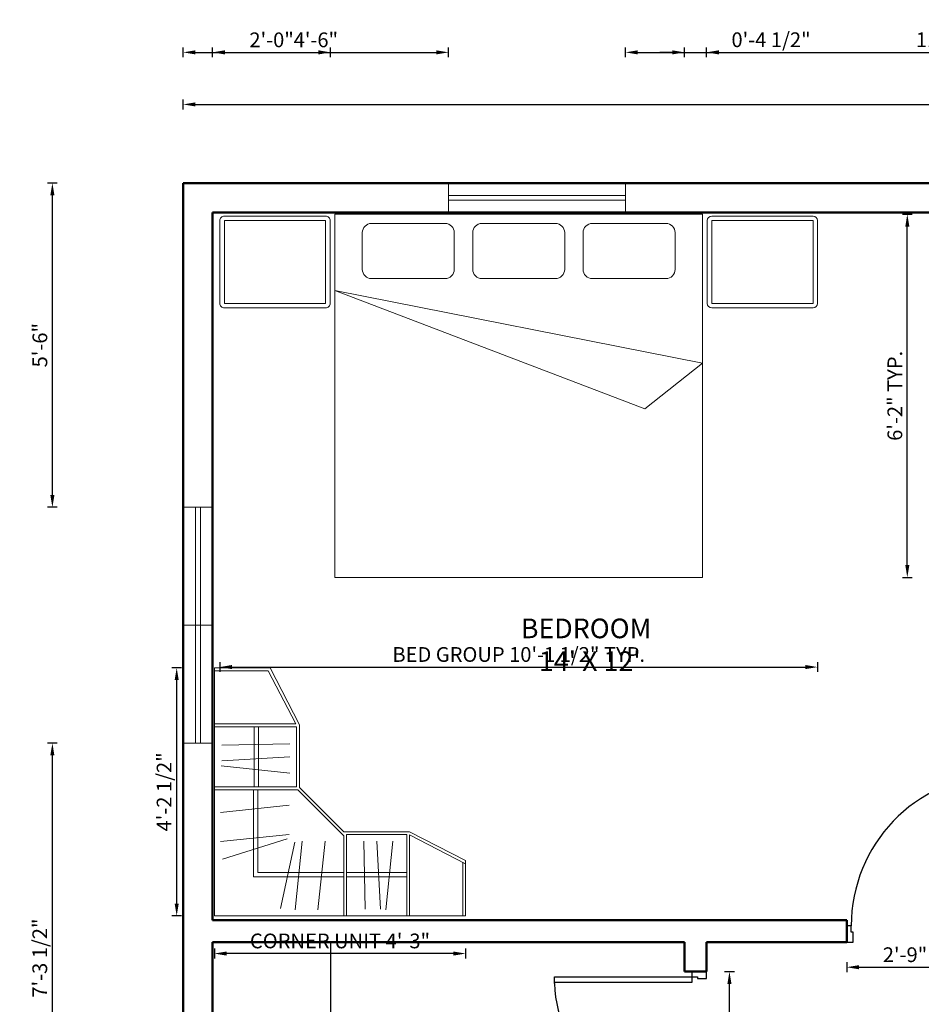
# Model space of a CAD drawing. Units: inches. Extents: x 1961 to 3038, y 800 to 1438.
# Tile 11 of 13: x 2592 to 2775, y 1148 to 1348. Entities that reach past the tile are written whole.
import ezdxf

# ---------------------------------------------------------------- set-up
doc = ezdxf.new("R2010")
doc.units = ezdxf.units.IN
for name, color, linetype, lineweight in [('A-ANNO-DIMS', 2, 'Continuous', 18), ('A-AREA-IDEN', 7, 'Continuous', 25), ('A-DOOR', 3, 'Continuous', 25), ('A-FLOR-CASE', 8, 'Continuous', 25), ('A-FURN', 8, 'Continuous', 18), ('A-GLAZ', 4, 'Continuous', 18), ('A-WALL', 7, 'Continuous', 50)]:
    doc.layers.add(name, color=color, linetype=linetype, lineweight=lineweight)
doc.styles.get("Standard").update_dxf_attribs({"font": 'arial.ttf'})
doc.dimstyles.new('ISO-25', dxfattribs={"dimtxt": 3, "dimasz": 2.5, "dimexe": 1, "dimexo": 1, "dimtad": 1, "dimdec": 4, "dimlunit": 4, "dimtxsty": 'Standard', "dimcen": 2.5, "dimadec": 0, "dimazin": 0, "dimtfac": 1, "dimtdec": 4, "dimtmove": 0, "dimatfit": 3, "dimfxl": 1, "dimfxlon": 1, "dimarcsym": 0})

# ---------------------------------------------------------------- blocks, each defined once
blk = doc.blocks.new('door 26')
for p, q in [((2685.19, 1125.64), (2685.19, 1127.01)), ((2685.19, 1127.01), (2713.13, 1127.01)), ((2713.13, 1128.04), (2713.13, 1125.8)), ((2713.13, 1127.01), (2714.34, 1127.01)), ((2714.34, 1127.01), (2714.34, 1126.64)), ((2714.34, 1126.64), (2716.17, 1126.64)), ((2716.17, 1126.64), (2716.17, 1128.04)), ((2713.13, 1125.8), (2685.19, 1125.8))]:
    blk.add_line(p, q)
blk.add_lwpolyline([(2716.17, 1098.04), (2716.17, 1099.26), (2714.34, 1099.26), (2714.34, 1098.89), (2713.13, 1098.89), (2713.13, 1098.04)])
blk.add_arc((2713.13, 1126.85), 27.97, 182.4896, 270)
blk = doc.blocks.new('A$C793B20D3')
for p, q in [((0.575, 1.9405), (0.025, 1.9405)), ((0.025, 1.9405), (0.025, 1.4905)), ((0.575, 1.4905), (0.575, 1.9405)), ((0.625, 0), (0.625, 1.975)), ((2.625, 1.975), (0.625, 1.975)), ((2.625, 0), (2.625, 1.975)), ((2.65, 1.4905), (2.65, 1.9405)), ((2.675, 1.9655), (3.225, 1.9655)), ((3.25, 1.9405), (3.25, 1.4905)), ((0.775, 1.675), (0.775, 1.875)), ((0.825, 1.925), (1.225, 1.925)), ((1.275, 1.675), (1.275, 1.875)), ((1.375, 1.675), (1.375, 1.875)), ((1.425, 1.925), (1.825, 1.925)), ((1.875, 1.675), (1.875, 1.875)), ((1.975, 1.675), (1.975, 1.875)), ((2.025, 1.925), (2.425, 1.925)), ((2.475, 1.675), (2.475, 1.875)), ((0.825, 1.625), (1.225, 1.625)), ((1.425, 1.625), (1.825, 1.625)), ((2.025, 1.625), (2.425, 1.625)), ((0.6256, 1.5604), (2.3107, 0.9169)), ((0.6256, 1.5604), (2.625, 1.1646)), ((0.025, 1.4905), (0.575, 1.4905)), ((3.225, 1.4655), (2.675, 1.4655)), ((2.3107, 0.9169), (2.625, 1.1646)), ((2.625, 0), (0.625, 0))]:
    blk.add_line(p, q)
at = {"flags": 128}
blk.add_lwpolyline([(0, 1.9405), (0, 1.4905, 0.414214), (0.025, 1.4655), (0.575, 1.4655, 0.414214), (0.6, 1.4905), (0.6, 1.9405, 0.414214), (0.575, 1.9655), (0.025, 1.9655, 0.414214)], format="xyb", close=True, dxfattribs=at)
blk.add_lwpolyline([(3.225, 1.9405), (3.225, 1.4905), (2.675, 1.4905), (2.675, 1.9405)], close=True)
for centre, radius, start, end in [((2.675, 1.9405), 0.025, 90, 180), ((3.225, 1.9405), 0.025, 0, 90), ((0.825, 1.875), 0.05, 90, 180), ((1.225, 1.875), 0.05, 0, 90), ((1.425, 1.875), 0.05, 90, 180), ((1.825, 1.875), 0.05, 0, 90), ((2.025, 1.875), 0.05, 90, 180), ((2.425, 1.875), 0.05, 0, 90), ((0.825, 1.675), 0.05, 180, 270), ((1.225, 1.675), 0.05, 270, 0), ((1.425, 1.675), 0.05, 180, 270), ((1.825, 1.675), 0.05, 270, 0), ((2.025, 1.675), 0.05, 180, 270), ((2.425, 1.675), 0.05, 270, 0), ((2.675, 1.4905), 0.025, 180, 270), ((3.225, 1.4905), 0.025, 270, 0)]:
    blk.add_arc(centre, radius, start, end)
blk = doc.blocks.new('A$C379C348A')
for p, q in [((1186.4, 1363.9), (1396.2, 1771)), ((1396.2, 1771), (1793.4, 1771)), ((1793.4, 1771), (1793.4, 0)), ((1212.5, 1371), (1408.4, 1751)), ((1408.4, 1751), (1793.4, 1751)), ((1186.4, 917.4), (1186.4, 1363.9)), ((1206.4, 1351), (1793.4, 1351)), ((1206.4, 921), (1206.4, 1351)), ((1212.5, 1371), (1793.4, 1371)), ((1479, 921.6), (1479, 1351.6)), ((1509.8, 921.6), (1509.8, 1351.6)), ((1255.5, 1228.5), (1740.8, 1219.3)), ((1740.8, 1108.3), (1255.5, 1136)), ((1255.5, 1020.4), (1745.4, 1071.2)), ((870, 601), (1186.4, 917.4)), ((1206.4, 921), (1793.4, 921)), ((870, 572.7), (1198.3, 901)), ((1198.3, 901), (1793.4, 901)), ((1483.9, 901), (1484.1, 309.1)), ((1514.7, 901), (1514.9, 278.3)), ((1260.4, 789.5), (1750.4, 738.8)), ((0, 394.8), (400, 601)), ((0, 372.3), (400, 578.5)), ((850, 601), (400, 601)), ((400, 578.5), (400, 0)), ((420, 581), (420, 0)), ((850, 581), (420, 581)), ((850, 601), (870, 601)), ((850, 581), (850, 0)), ((870, 572.7), (870, 0)), ((1260.5, 581.2), (1750.5, 530.6)), ((518.8, 532.6), (569.6, 42.7)), ((606.7, 47.3), (634.4, 532.6)), ((726.9, 532.6), (717.7, 47.3)), ((1003.7, 532.6), (1054.5, 42.7)), ((1166.2, 532.6), (1217.1, 42.7)), ((1321.2, 51.6), (1217.9, 526.5)), ((1736.6, 405.8), (1272.7, 550.9)), ((0, 394.8), (0, 0)), ((20, 382.7), (20, 0)), ((420, 309.1), (850, 309.1)), ((870, 309.1), (1484.1, 309.1)), ((420, 278.3), (850, 278.3)), ((870, 278.3), (1514.9, 278.3)), ((0, 0), (1793.4, 0))]:
    blk.add_line(p, q)
blk = doc.blocks.new('*D25')
at = {"layer": 'A-ANNO-DIMS', "color": 0, "lineweight": -2, "transparency": 16777216}
for p, q in [((2624.77, 1329.92), (2624.77, 1331.92)), ((2627.27, 1330.92), (3006.27, 1330.92)), ((3008.77, 1329.92), (3008.77, 1331.92))]:
    blk.add_line(p, q, dxfattribs=at)
at = {"layer": 'A-ANNO-DIMS', "color": 0, "transparency": 16777216}
for points in [[(2627.27, 1331.34), (2627.27, 1330.51), (2624.77, 1330.92)], [(3006.27, 1331.34), (3006.27, 1330.51), (3008.77, 1330.92)]]:
    blk.add_solid(points, dxfattribs=at)
at = {"layer": 'Defpoints', "color": 0, "transparency": 16777216}
for p in [(3008.77, 1330.92), (2624.77, 1314.92), (3008.77, 1314.92)]:
    blk.add_point(p, dxfattribs=at)
at = {"layer": 'A-ANNO-DIMS', "color": 0, "transparency": 16777216, "insert": (2816.77, 1333.08), "char_height": 3, "attachment_point": 5}
blk.add_mtext("32'", dxfattribs=at)
blk = doc.blocks.new('WIN-36IN')
for p, q in [((0, 36), (6, 36)), ((2.5, 36), (2.5, 0)), ((3.5, 36), (3.5, 0)), ((0, 0), (6, 0))]:
    blk.add_line(p, q)
blk = doc.blocks.new('WIN-48IN-MULLION')
for p, q in [((6, 48), (0, 48)), ((2.5, 48), (2.5, 0)), ((3.5, 48), (3.5, 0)), ((6, 24), (0, 24)), ((6, 0), (0, 0))]:
    blk.add_line(p, q)
blk = doc.blocks.new('DOOR-SWING-33IN')
for p, q in [((30.36, 34.07), (31.87, 34.07)), ((30.53, 3.34), (30.53, 34.07)), ((31.87, 34.07), (31.87, 3.34)), ((33, 3.34), (30.53, 3.34)), ((31.87, 2), (31.46, 2)), ((31.46, 2), (31.46, 0)), ((31.87, 3.34), (31.87, 2)), ((31.46, 0), (33, 0))]:
    blk.add_line(p, q)
blk.add_lwpolyline([(0, 0), (1.34, 0), (1.34, 2), (0.93, 2), (0.93, 3.34), (0, 3.34)])
blk.add_arc((31.69, 3.34), 30.76, 92.4896, 180)
blk = doc.blocks.new('*D37')
at = {"layer": 'A-ANNO-DIMS', "color": 0, "lineweight": -2, "transparency": 16777216}
for p, q in [((2632.21, 1217.4), (2632.21, 1215.4)), ((2753.86, 1217.4), (2753.86, 1215.4)), ((2634.71, 1216.4), (2751.36, 1216.4))]:
    blk.add_line(p, q, dxfattribs=at)
at = {"layer": 'A-ANNO-DIMS', "color": 0, "transparency": 16777216}
for points in [[(2634.71, 1216.82), (2634.71, 1215.99), (2632.21, 1216.4)], [(2751.36, 1216.82), (2751.36, 1215.99), (2753.86, 1216.4)]]:
    blk.add_solid(points, dxfattribs=at)
at = {"layer": 'Defpoints', "color": 0, "transparency": 16777216}
for p in [(2632.21, 1234.65), (2753.86, 1234.65), (2753.86, 1216.4)]:
    blk.add_point(p, dxfattribs=at)
at = {"layer": 'A-ANNO-DIMS', "color": 0, "transparency": 16777216, "insert": (2693.04, 1218.58), "char_height": 3, "attachment_point": 5}
blk.add_mtext('BED GROUP 10\'-1 1/2" TYP.', dxfattribs=at)
blk = doc.blocks.new('*D38')
at = {"layer": 'A-ANNO-DIMS', "color": 0, "lineweight": -2, "transparency": 16777216}
for p, q in [((2771.1, 1308.57), (2773.1, 1308.57)), ((2772.1, 1237.15), (2772.1, 1306.07)), ((2771.1, 1234.65), (2773.1, 1234.65))]:
    blk.add_line(p, q, dxfattribs=at)
at = {"layer": 'A-ANNO-DIMS', "color": 0, "transparency": 16777216}
for points in [[(2771.69, 1306.07), (2772.52, 1306.07), (2772.1, 1308.57)], [(2771.69, 1237.15), (2772.52, 1237.15), (2772.1, 1234.65)]]:
    blk.add_solid(points, dxfattribs=at)
at = {"layer": 'Defpoints', "color": 0, "transparency": 16777216}
for p in [(2753.86, 1308.57), (2772.1, 1308.57), (2753.86, 1234.65)]:
    blk.add_point(p, dxfattribs=at)
at = {"layer": 'A-ANNO-DIMS', "color": 0, "transparency": 16777216, "insert": (2769.95, 1271.61), "char_height": 3, "attachment_point": 5, "rotation": 90}
blk.add_mtext('6\'-2" TYP.', dxfattribs=at)
blk = doc.blocks.new('*D48')
at = {"layer": 'A-ANNO-DIMS', "color": 0, "lineweight": -2, "transparency": 16777216}
for p, q in [((2759.77, 1156.31), (2759.77, 1154.31)), ((2762.27, 1155.31), (2790.27, 1155.31)), ((2792.77, 1156.31), (2792.77, 1154.31))]:
    blk.add_line(p, q, dxfattribs=at)
at = {"layer": 'A-ANNO-DIMS', "color": 0, "transparency": 16777216}
for points in [[(2762.27, 1155.73), (2762.27, 1154.89), (2759.77, 1155.31)], [(2790.27, 1155.73), (2790.27, 1154.89), (2792.77, 1155.31)]]:
    blk.add_solid(points, dxfattribs=at)
at = {"layer": 'Defpoints', "color": 0, "transparency": 16777216}
for p in [(2759.77, 1160.42), (2792.77, 1160.42), (2792.77, 1155.31)]:
    blk.add_point(p, dxfattribs=at)
at = {"layer": 'A-ANNO-DIMS', "color": 0, "transparency": 16777216, "insert": (2776.27, 1157.47), "char_height": 3, "attachment_point": 5}
blk.add_mtext('2\'-9" TYP.', dxfattribs=at)
blk = doc.blocks.new('*D52')
at = {"layer": 'A-ANNO-DIMS', "color": 0, "lineweight": -2, "transparency": 16777216}
for p, q in [((2734.91, 1154.42), (2736.91, 1154.42)), ((2735.91, 1126.92), (2735.91, 1151.92)), ((2734.91, 1124.42), (2736.91, 1124.42))]:
    blk.add_line(p, q, dxfattribs=at)
at = {"layer": 'A-ANNO-DIMS', "color": 0, "transparency": 16777216}
for points in [[(2735.5, 1151.92), (2736.33, 1151.92), (2735.91, 1154.42)], [(2735.5, 1126.92), (2736.33, 1126.92), (2735.91, 1124.42)]]:
    blk.add_solid(points, dxfattribs=at)
at = {"layer": 'Defpoints', "color": 0, "transparency": 16777216}
for p in [(2731.27, 1154.42), (2735.91, 1154.42), (2731.27, 1124.42)]:
    blk.add_point(p, dxfattribs=at)
at = {"layer": 'A-ANNO-DIMS', "color": 0, "transparency": 16777216, "insert": (2733.76, 1139.42), "char_height": 3, "attachment_point": 5, "rotation": 90}
blk.add_mtext('2\'-6"', dxfattribs=at)
blk = doc.blocks.new('*D55')
at = {"layer": 'A-ANNO-DIMS', "color": 0, "lineweight": -2, "transparency": 16777216}
for p, q in [((2631.13, 1159.09), (2631.13, 1157.09)), ((2682.24, 1159.09), (2682.24, 1157.09)), ((2679.74, 1158.09), (2633.63, 1158.09))]:
    blk.add_line(p, q, dxfattribs=at)
at = {"layer": 'A-ANNO-DIMS', "color": 0, "transparency": 16777216}
for points in [[(2633.63, 1158.51), (2633.63, 1157.68), (2631.13, 1158.09)], [(2679.74, 1158.51), (2679.74, 1157.68), (2682.24, 1158.09)]]:
    blk.add_solid(points, dxfattribs=at)
at = {"layer": 'Defpoints', "color": 0, "transparency": 16777216}
for p in [(2631.13, 1165.76), (2682.24, 1165.76), (2631.13, 1158.09)]:
    blk.add_point(p, dxfattribs=at)
at = {"layer": 'A-ANNO-DIMS', "color": 0, "transparency": 16777216, "insert": (2656.68, 1160.27), "char_height": 3, "attachment_point": 5}
blk.add_mtext('CORNER UNIT 4\'-3"', dxfattribs=at)
blk = doc.blocks.new('*D56')
at = {"layer": 'A-ANNO-DIMS', "color": 0, "lineweight": -2, "transparency": 16777216}
for p, q in [((2624.46, 1216.24), (2622.46, 1216.24)), ((2623.46, 1168.26), (2623.46, 1213.74)), ((2624.46, 1165.76), (2622.46, 1165.76))]:
    blk.add_line(p, q, dxfattribs=at)
at = {"layer": 'A-ANNO-DIMS', "color": 0, "transparency": 16777216}
for points in [[(2623.04, 1213.74), (2623.87, 1213.74), (2623.46, 1216.24)], [(2623.04, 1168.26), (2623.87, 1168.26), (2623.46, 1165.76)]]:
    blk.add_solid(points, dxfattribs=at)
at = {"layer": 'Defpoints', "color": 0, "transparency": 16777216}
for p in [(2623.46, 1216.24), (2631.13, 1216.24), (2631.13, 1165.76)]:
    blk.add_point(p, dxfattribs=at)
at = {"layer": 'A-ANNO-DIMS', "color": 0, "transparency": 16777216, "insert": (2621.28, 1191), "char_height": 3, "attachment_point": 5, "rotation": 90}
blk.add_mtext('4\'-2 1/2"', dxfattribs=at)
blk = doc.blocks.new('*D76')
at = {"layer": 'A-ANNO-DIMS', "color": 0, "lineweight": -2, "transparency": 16777216}
for p, q in [((2624.77, 1340.52), (2624.77, 1342.52)), ((2627.27, 1341.52), (2676.27, 1341.52)), ((2678.77, 1340.52), (2678.77, 1342.52))]:
    blk.add_line(p, q, dxfattribs=at)
at = {"layer": 'A-ANNO-DIMS', "color": 0, "transparency": 16777216}
for points in [[(2627.27, 1341.94), (2627.27, 1341.1), (2624.77, 1341.52)], [(2676.27, 1341.94), (2676.27, 1341.1), (2678.77, 1341.52)]]:
    blk.add_solid(points, dxfattribs=at)
at = {"layer": 'Defpoints', "color": 0, "transparency": 16777216}
for p in [(2678.77, 1341.52), (2624.77, 1314.92), (2678.77, 1314.92)]:
    blk.add_point(p, dxfattribs=at)
at = {"layer": 'A-ANNO-DIMS', "color": 0, "transparency": 16777216, "insert": (2651.77, 1343.68), "char_height": 3, "attachment_point": 5}
blk.add_mtext('4\'-6"', dxfattribs=at)
blk = doc.blocks.new('*D77')
at = {"layer": 'A-ANNO-DIMS', "color": 0, "lineweight": -2, "transparency": 16777216}
for p, q in [((2714.77, 1340.52), (2714.77, 1342.52)), ((2717.27, 1341.52), (2848.77, 1341.52)), ((2851.27, 1340.52), (2851.27, 1342.52))]:
    blk.add_line(p, q, dxfattribs=at)
at = {"layer": 'A-ANNO-DIMS', "color": 0, "transparency": 16777216}
for points in [[(2717.27, 1341.94), (2717.27, 1341.1), (2714.77, 1341.52)], [(2848.77, 1341.94), (2848.77, 1341.1), (2851.27, 1341.52)]]:
    blk.add_solid(points, dxfattribs=at)
at = {"layer": 'Defpoints', "color": 0, "transparency": 16777216}
for p in [(2851.27, 1341.52), (2714.77, 1314.92), (2851.27, 1314.92)]:
    blk.add_point(p, dxfattribs=at)
at = {"layer": 'A-ANNO-DIMS', "color": 0, "transparency": 16777216, "insert": (2783.02, 1343.7), "char_height": 3, "attachment_point": 5}
blk.add_mtext('11\'-4 1/2"', dxfattribs=at)
blk = doc.blocks.new('*D79')
at = {"layer": 'A-ANNO-DIMS', "color": 0, "lineweight": -2, "transparency": 16777216}
for p, q in [((2599.17, 1314.92), (2597.17, 1314.92)), ((2598.17, 1251.42), (2598.17, 1312.42)), ((2599.17, 1248.92), (2597.17, 1248.92))]:
    blk.add_line(p, q, dxfattribs=at)
at = {"layer": 'A-ANNO-DIMS', "color": 0, "transparency": 16777216}
for points in [[(2597.75, 1312.42), (2598.58, 1312.42), (2598.17, 1314.92)], [(2597.75, 1251.42), (2598.58, 1251.42), (2598.17, 1248.92)]]:
    blk.add_solid(points, dxfattribs=at)
at = {"layer": 'Defpoints', "color": 0, "transparency": 16777216}
for p in [(2598.17, 1314.92), (2624.77, 1314.92), (2624.77, 1248.92)]:
    blk.add_point(p, dxfattribs=at)
at = {"layer": 'A-ANNO-DIMS', "color": 0, "transparency": 16777216, "insert": (2596.01, 1281.92), "char_height": 3, "attachment_point": 5, "rotation": 90}
blk.add_mtext('5\'-6"', dxfattribs=at)
blk = doc.blocks.new('*D80')
at = {"layer": 'A-ANNO-DIMS', "color": 0, "lineweight": -2, "transparency": 16777216}
for p, q in [((2599.17, 1200.92), (2597.17, 1200.92)), ((2598.17, 1115.92), (2598.17, 1198.42)), ((2599.17, 1113.42), (2597.17, 1113.42))]:
    blk.add_line(p, q, dxfattribs=at)
at = {"layer": 'A-ANNO-DIMS', "color": 0, "transparency": 16777216}
for points in [[(2597.75, 1198.42), (2598.58, 1198.42), (2598.17, 1200.92)], [(2597.75, 1115.92), (2598.58, 1115.92), (2598.17, 1113.42)]]:
    blk.add_solid(points, dxfattribs=at)
at = {"layer": 'Defpoints', "color": 0, "transparency": 16777216}
for p in [(2598.17, 1200.92), (2624.77, 1200.92), (2624.77, 1113.42)]:
    blk.add_point(p, dxfattribs=at)
at = {"layer": 'A-ANNO-DIMS', "color": 0, "transparency": 16777216, "insert": (2595.99, 1157.17), "char_height": 3, "attachment_point": 5, "rotation": 90}
blk.add_mtext('7\'-3 1/2"', dxfattribs=at)
blk = doc.blocks.new('*D86')
at = {"layer": 'A-ANNO-DIMS', "color": 0, "lineweight": -2, "transparency": 16777216}
for p, q in [((2630.77, 1340.52), (2630.77, 1342.52)), ((2633.27, 1341.52), (2652.27, 1341.52)), ((2654.77, 1340.52), (2654.77, 1342.52))]:
    blk.add_line(p, q, dxfattribs=at)
at = {"layer": 'A-ANNO-DIMS', "color": 0, "transparency": 16777216}
for points in [[(2633.27, 1341.94), (2633.27, 1341.1), (2630.77, 1341.52)], [(2652.27, 1341.94), (2652.27, 1341.1), (2654.77, 1341.52)]]:
    blk.add_solid(points, dxfattribs=at)
at = {"layer": 'Defpoints', "color": 0, "transparency": 16777216}
for p in [(2654.77, 1341.52), (2630.77, 1160.42), (2654.77, 1160.42)]:
    blk.add_point(p, dxfattribs=at)
at = {"layer": 'A-ANNO-DIMS', "color": 0, "transparency": 16777216, "insert": (2642.77, 1343.68), "char_height": 3, "attachment_point": 5}
blk.add_mtext('2\'-0"', dxfattribs=at)
blk = doc.blocks.new('*D91')
at = {"layer": 'A-ANNO-DIMS', "color": 0, "lineweight": -2, "transparency": 16777216}
for p, q in [((2724.27, 1341.52), (2721.77, 1341.52)), ((2726.77, 1340.52), (2726.77, 1342.52)), ((2726.77, 1341.52), (2731.27, 1341.52)), ((2731.27, 1340.52), (2731.27, 1342.52)), ((2733.77, 1341.52), (2752.48, 1341.52))]:
    blk.add_line(p, q, dxfattribs=at)
at = {"layer": 'A-ANNO-DIMS', "color": 0, "transparency": 16777216}
for points in [[(2724.27, 1341.94), (2724.27, 1341.1), (2726.77, 1341.52)], [(2733.77, 1341.94), (2733.77, 1341.1), (2731.27, 1341.52)]]:
    blk.add_solid(points, dxfattribs=at)
at = {"layer": 'Defpoints', "color": 0, "transparency": 16777216}
for p in [(2731.27, 1341.52), (2726.77, 1160.42), (2731.27, 1160.42)]:
    blk.add_point(p, dxfattribs=at)
at = {"layer": 'A-ANNO-DIMS', "color": 0, "transparency": 16777216, "insert": (2744.38, 1343.7), "char_height": 3, "attachment_point": 5}
blk.add_mtext('0\'-4 1/2"', dxfattribs=at)

msp = doc.modelspace()

# ---------------------------------------------------------------- linework, layer by layer
at = {"layer": 'A-FLOR-CASE'}
msp.add_line((2654.76803, 1160.41975), (2654.76803, 1082.41975), dxfattribs=at)
at = {"layer": 'A-WALL'}
for p, q in [((3008.76803, 1314.91975), (2624.76803, 1314.91975)), ((2624.76803, 1314.91975), (2624.76803, 852.91975)), ((2630.76803, 1308.91975), (2630.76803, 1164.91975)), ((2798.76803, 1308.91975), (2630.76803, 1308.91975)), ((2759.76803, 1164.91975), (2630.76803, 1164.91975)), ((2759.76803, 1164.91975), (2759.76803, 1160.41975)), ((2726.76803, 1160.41975), (2630.76803, 1160.41975)), ((2630.76803, 1160.41975), (2630.76803, 1058.41975)), ((2726.76803, 1160.41975), (2726.76803, 1154.41975)), ((2731.26803, 1160.41975), (2731.26803, 1154.41975)), ((2759.76803, 1160.41975), (2731.26803, 1160.41975)), ((2731.26803, 1154.41975), (2726.76803, 1154.41975))]:
    msp.add_line(p, q, dxfattribs=at)

# ---------------------------------------------------------------- block references
at = {"layer": 'A-DOOR'}
for name, p in [('DOOR-SWING-33IN', (2759.768, 1160.42)), ('door 26', (15.10265, 26.37719))]:
    msp.add_blockref(name, p, dxfattribs=at)
at = {"layer": 'A-FURN'}
for name, p, xscale, yscale, zscale in [('A$C793B20D3', (2632.21469, 1234.64816), 37.42822407468409, 37.42822407468409, 37.42822407468409), ('A$C379C348A', (2682.23715, 1165.76029), -0.0285003206593903, 0.0285003206593903, 0.0285003206593903)]:
    msp.add_blockref(name, p, dxfattribs=dict(at, xscale=xscale, yscale=yscale, zscale=zscale))
at = {"layer": 'A-GLAZ', "rotation": 90.000000000003}
msp.add_blockref('WIN-36IN', (2714.76779, 1308.91972), dxfattribs=at)
at = {"layer": 'A-GLAZ'}
msp.add_blockref('WIN-48IN-MULLION', (2624.768, 1200.92), dxfattribs=at)

# ---------------------------------------------------------------- texts
at = {"layer": 'A-AREA-IDEN', "insert": (2693.48089, 1226.27259), "char_height": 4, "attachment_point": 1}
msp.add_mtext_dynamic_manual_height_columns("{\\fTimes New Roman|b1|i0|c0|p18;BEDROOM\\P   14' X 12'}", width=33.1080891, gutter_width=12.5, heights=[0], dxfattribs=at)

# ---------------------------------------------------------------- dimensions: what is measured, and where the dimension line sits
at = {"layer": 'A-ANNO-DIMS'}
for base, p1, p2, override, picture, middle in [((2851.26803, 1341.51975), (2714.76803, 1314.91975), (2851.26803, 1314.91975), {"dimdec": 1, "dimlfac": 1, "dimrnd": 0, "dimzin": 1, "dimdsep": 46, "dimlunit": 4, "dimfrac": 2}, '*D77', (2783.01803, 1343.69591)), ((2731.26803, 1341.51975), (2726.76803, 1160.41975), (2731.26803, 1160.41975), {"dimdec": 1, "dimlfac": 1, "dimrnd": 0, "dimzin": 1, "dimdsep": 46, "dimlunit": 4, "dimfrac": 2}, '*D91', (2744.37564, 1343.69591)), ((2678.76803, 1341.51975), (2624.76803, 1314.91975), (2678.76803, 1314.91975), {"dimdec": 1, "dimlfac": 1, "dimrnd": 0, "dimzin": 1, "dimdsep": 46, "dimlunit": 4, "dimfrac": 2}, '*D76', (2651.76803, 1343.67647)), ((2654.76803, 1341.51975), (2630.76803, 1160.41975), (2654.76803, 1160.41975), {"dimdec": 1, "dimlfac": 1, "dimrnd": 0, "dimzin": 1, "dimdsep": 46, "dimlunit": 4, "dimfrac": 2}, '*D86', (2642.76803, 1343.67647)), ((3008.76803, 1330.92264), (2624.76803, 1314.91975), (3008.76803, 1314.91975), {"dimclrd": 0, "dimclre": 0, "dimclrt": 0}, '*D25', (2816.76803, 1333.08038))]:
    dim = msp.add_linear_dim(base=base, p1=p1, p2=p2, dimstyle='ISO-25', override=override, dxfattribs=at)
    dim.commit()
    dim.dimension.update_dxf_attribs({"geometry": picture, "text_midpoint": middle})
for base, p1, p2, picture, middle in [((2598.16803, 1314.91975), (2624.76803, 1248.91975), (2624.76803, 1314.91975), '*D79', (2596.01131, 1281.91975)), ((2623.45827, 1216.23504), (2631.12508, 1165.76029), (2631.12508, 1216.23504), '*D56', (2621.28211, 1190.99767)), ((2598.16803, 1200.91975), (2624.76803, 1113.41975), (2624.76803, 1200.91975), '*D80', (2595.99085, 1157.16975)), ((2735.91454, 1154.41975), (2731.26803, 1124.41975), (2731.26803, 1154.41975), '*D52', (2733.75783, 1139.41975))]:
    dim = msp.add_linear_dim(base=base, p1=p1, p2=p2, angle=90, dimstyle='ISO-25', override={"dimdec": 1, "dimlfac": 1, "dimrnd": 0, "dimzin": 1, "dimdsep": 46, "dimlunit": 4, "dimfrac": 2}, dxfattribs=at)
    dim.commit()
    dim.dimension.update_dxf_attribs({"geometry": picture, "text_midpoint": middle})
for base, p1, p2, angle, text, picture, middle in [((2772.10288, 1308.56907), (2753.85662, 1234.64833), (2753.85662, 1308.56907), 90, '<> TYP.', '*D38', (2769.94616, 1271.6087)), ((2631.12508, 1158.09348), (2682.23715, 1165.76029), (2631.12508, 1165.76029), 180, 'CORNER UNIT <>', '*D55', (2656.68111, 1160.27169))]:
    dim = msp.add_linear_dim(base=base, p1=p1, p2=p2, angle=angle, text=text, dimstyle='ISO-25', override={"dimdec": 1, "dimlfac": 1, "dimrnd": 0, "dimzin": 1, "dimdsep": 46, "dimlunit": 4, "dimfrac": 2}, dxfattribs=at)
    dim.commit()
    dim.dimension.update_dxf_attribs({"geometry": picture, "text_midpoint": middle})
for base, p1, p2, text, picture, middle in [((2753.85662, 1216.40207), (2632.21489, 1234.64833), (2753.85662, 1234.64833), 'BED GROUP <> TYP.', '*D37', (2693.03575, 1218.57925)), ((2792.76803, 1155.30859), (2759.76803, 1160.41975), (2792.76803, 1160.41975), '<> TYP.', '*D48', (2776.26803, 1157.46531))]:
    dim = msp.add_linear_dim(base=base, p1=p1, p2=p2, text=text, dimstyle='ISO-25', override={"dimdec": 1, "dimlfac": 1, "dimrnd": 0, "dimzin": 1, "dimdsep": 46, "dimlunit": 4, "dimfrac": 2}, dxfattribs=at)
    dim.commit()
    dim.dimension.update_dxf_attribs({"geometry": picture, "text_midpoint": middle})

doc.saveas('drawing.dxf')
